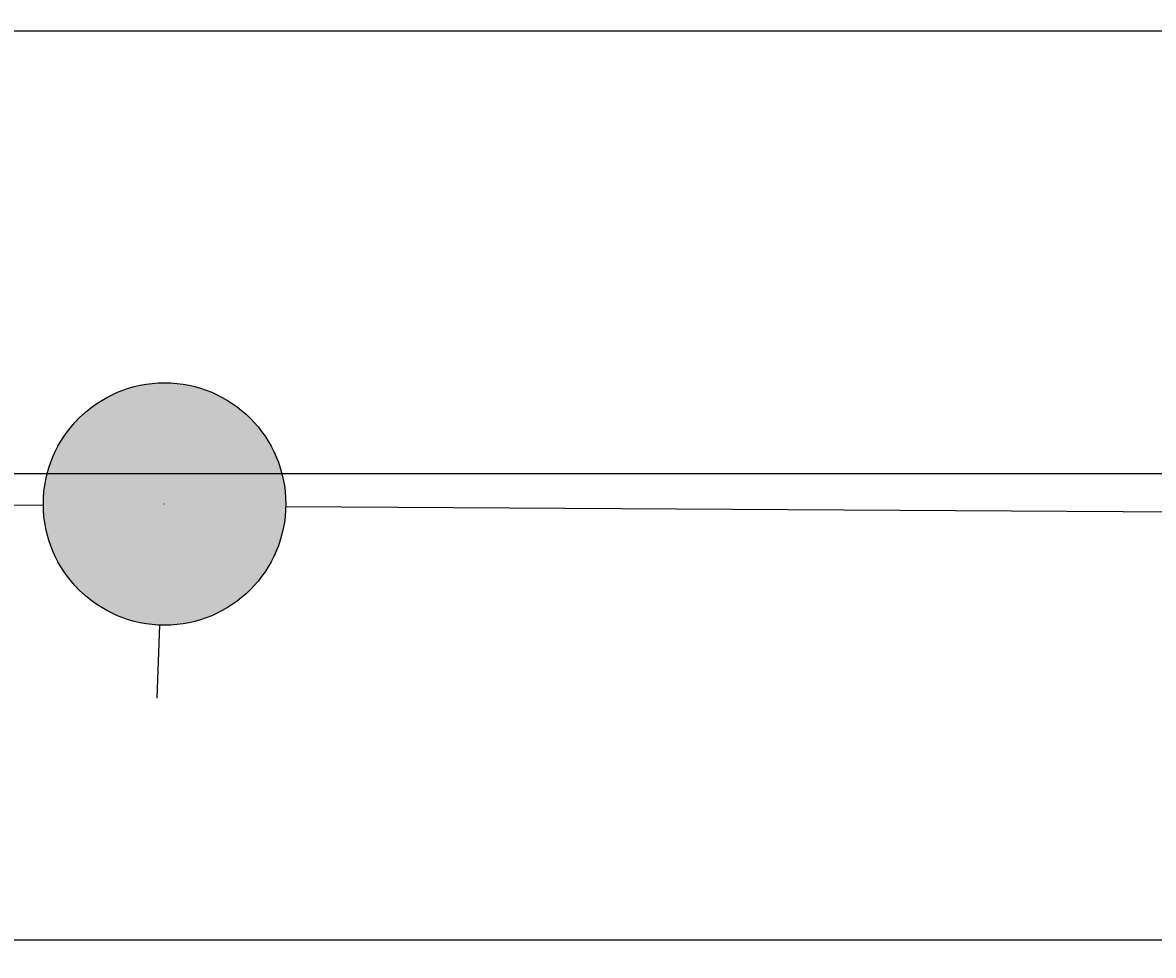
# Model space of a CAD drawing. Units: inches. Extents: x 35362 to 73946, y 43607 to 67532.
# Tile 10 of 134: x 42029 to 43509, y 47688 to 48909. Entities that reach past the tile are written whole.
import ezdxf

# ---------------------------------------------------------------- set-up
doc = ezdxf.new("R2010")
doc.units = ezdxf.units.IN
doc.header["$MEASUREMENT"] = 0
for name, color, linetype, lineweight in [('A-ANNO-DIMS', 2, 'Continuous', 18), ('E-SYMB', 1, 'Continuous', 25), ('E-SYMB-PATT', 1, 'Continuous', 13), ('E-WIRE', 3, 'Continuous', 25)]:
    doc.layers.add(name, color=color, linetype=linetype, lineweight=lineweight)
doc.styles.get("Standard").update_dxf_attribs({"font": 'arial.ttf'})
doc.dimstyles.get("Standard").update_dxf_attribs({"dimtxt": 0.18, "dimasz": 0.18, "dimexe": 0.18, "dimexo": 0.0625, "dimgap": 0.09, "dimtad": 0, "dimtih": 1, "dimtoh": 1, "dimdec": 4, "dimzin": 0, "dimdsep": 46, "dimtxsty": 'Standard', "dimcen": 0.09, "dimadec": 0, "dimazin": 0, "dimtfac": 1, "dimtdec": 4, "dimtofl": 0, "dimtmove": 0, "dimatfit": 3, "dimfxl": 1, "dimtolj": 1, "dimtzin": 0, "dimarcsym": 0})

# ---------------------------------------------------------------- blocks, each defined once
blk = doc.blocks.new('*D21')
at = {"layer": 'A-ANNO-DIMS', "color": 0, "lineweight": -2, "transparency": 16777216}
for p, q in [((42214.5, 48279), (42214.7, 48279)), ((42214.6, 48278.9), (42214.6, 48279.1)), ((42204.8, 48025.4), (42208.5, 48120.3)), ((42204.7, 48025.4), (42204.8, 48025.4))]:
    blk.add_line(p, q, dxfattribs=at)
at = {"layer": 'A-ANNO-DIMS', "color": 0, "transparency": 16777216}
blk.add_solid([(42208.5, 48120.3), (42208.5, 48120.3), (42208.5, 48120.5)], dxfattribs=at)
at = {"layer": 'Defpoints', "color": 0, "transparency": 16777216}
for p in [(42220.8, 48437.5), (42208.5, 48120.5)]:
    blk.add_point(p, dxfattribs=at)
at = {"layer": 'A-ANNO-DIMS', "color": 0, "transparency": 16777216, "insert": (42203.9, 48025.4), "char_height": 0.18, "attachment_point": 5}
blk.add_mtext('\\A1;26X ∅317.2', dxfattribs=at)
blk = doc.blocks.new('*D61')
at = {"layer": 'A-ANNO-DIMS', "color": 0, "lineweight": -2, "transparency": 16777216}
for p, q in [((42214.5, 48279), (42214.7, 48279)), ((42214.6, 48278.9), (42214.6, 48279.1)), ((42204.8, 48025.4), (42208.5, 48120.3)), ((42204.7, 48025.4), (42204.8, 48025.4))]:
    blk.add_line(p, q, dxfattribs=at)
at = {"layer": 'A-ANNO-DIMS', "color": 0, "transparency": 16777216}
blk.add_solid([(42208.5, 48120.3), (42208.5, 48120.3), (42208.5, 48120.5)], dxfattribs=at)
at = {"layer": 'Defpoints', "color": 0, "transparency": 16777216}
for p in [(42220.8, 48437.5), (42208.5, 48120.5)]:
    blk.add_point(p, dxfattribs=at)
at = {"layer": 'A-ANNO-DIMS', "color": 0, "transparency": 16777216, "insert": (42203.9, 48025.4), "char_height": 0.18, "attachment_point": 5}
blk.add_mtext('\\A1;26X ∅317.2', dxfattribs=at)
blk = doc.blocks.new('*D67')
at = {"layer": 'A-ANNO-DIMS', "color": 0, "lineweight": -2, "transparency": 16777216}
for p, q in [((56873.5, 53351.5), (35361.8, 53351.5)), ((35361.9, 53351.3), (35361.9, 49400.9)), ((35361.9, 45450.1), (35361.9, 49400.5)), ((53793.6, 45449.9), (35361.8, 45449.9))]:
    blk.add_line(p, q, dxfattribs=at)
at = {"layer": 'A-ANNO-DIMS', "color": 0, "transparency": 16777216}
for points in [[(35361.9, 53351.3), (35362, 53351.3), (35361.9, 53351.5)], [(35361.9, 45450.1), (35362, 45450.1), (35361.9, 45449.9)]]:
    blk.add_solid(points, dxfattribs=at)
at = {"layer": 'Defpoints', "color": 0, "transparency": 16777216}
for p in [(35361.9, 53351.5), (56873.6, 53351.5), (53793.6, 45449.9)]:
    blk.add_point(p, dxfattribs=at)
at = {"layer": 'A-ANNO-DIMS', "color": 0, "transparency": 16777216, "insert": (35361.9, 49400.7), "char_height": 0.18, "attachment_point": 5}
blk.add_mtext('\\A1;7901.6', dxfattribs=at)
blk = doc.blocks.new('*D87')
at = {"layer": 'A-ANNO-DIMS', "color": 0, "lineweight": -2, "transparency": 16777216}
for p, q in [((52362.5, 48318.3), (35361.8, 48318.3)), ((35361.9, 48318.1), (35361.9, 47931.4)), ((35361.9, 47544.3), (35361.9, 47931)), ((52362.5, 47544.1), (35361.8, 47544.1))]:
    blk.add_line(p, q, dxfattribs=at)
at = {"layer": 'A-ANNO-DIMS', "color": 0, "transparency": 16777216}
for points in [[(35361.9, 48318.1), (35362, 48318.1), (35361.9, 48318.3)], [(35361.9, 47544.3), (35362, 47544.3), (35361.9, 47544.1)]]:
    blk.add_solid(points, dxfattribs=at)
at = {"layer": 'Defpoints', "color": 0, "transparency": 16777216}
for p in [(35361.9, 48318.3), (52362.6, 48318.3), (52362.6, 47544.1)]:
    blk.add_point(p, dxfattribs=at)
at = {"layer": 'A-ANNO-DIMS', "color": 0, "transparency": 16777216, "insert": (35361.9, 47931.2), "char_height": 0.18, "attachment_point": 5}
blk.add_mtext('\\A1;774.1', dxfattribs=at)
blk = doc.blocks.new('*D89')
at = {"layer": 'A-ANNO-DIMS', "color": 0, "lineweight": -2, "transparency": 16777216}
for p, q in [((53707.7, 48897.7), (35361.8, 48897.7)), ((35361.9, 48897.6), (35361.9, 48303.2)), ((35361.9, 47708.4), (35361.9, 48302.8)), ((53707.7, 47708.2), (35361.8, 47708.2))]:
    blk.add_line(p, q, dxfattribs=at)
at = {"layer": 'A-ANNO-DIMS', "color": 0, "transparency": 16777216}
for points in [[(35361.9, 48897.6), (35362, 48897.6), (35361.9, 48897.7)], [(35361.9, 47708.4), (35362, 47708.4), (35361.9, 47708.2)]]:
    blk.add_solid(points, dxfattribs=at)
at = {"layer": 'Defpoints', "color": 0, "transparency": 16777216}
for p in [(53707.8, 48897.7), (35361.9, 47708.2), (53707.8, 47708.2)]:
    blk.add_point(p, dxfattribs=at)
at = {"layer": 'A-ANNO-DIMS', "color": 0, "transparency": 16777216, "insert": (35361.9, 48303), "char_height": 0.18, "attachment_point": 5}
blk.add_mtext('\\A1;1189.5', dxfattribs=at)

msp = doc.modelspace()

# ---------------------------------------------------------------- hatches: boundary and pattern name
at = {"layer": 'E-SYMB-PATT'}
h = msp.add_hatch(color=256, dxfattribs=at)
h.dxf.hatch_style = 1
h.paths.add_polyline_path([(42056.029, 48278.988, 1), (42373.241, 48278.988, 1)])
h = msp.add_hatch(color=256, dxfattribs=at)
h.dxf.hatch_style = 1
h.paths.add_polyline_path([(42373.206, 48275.646), (42056.036, 48277.555, 0.98505792)])

# ---------------------------------------------------------------- linework, layer by layer
at = {"layer": 'E-SYMB'}
msp.add_circle((42214.635, 48278.988), 158.606, dxfattribs=at)
at = {"layer": 'E-WIRE'}
for p, q in [((39894.84, 48290.562), (42056.036, 48277.555)), ((42373.206, 48275.646), (45390.147, 48257.489))]:
    msp.add_line(p, q, dxfattribs=at)

# ---------------------------------------------------------------- dimensions: what is measured, and where the dimension line sits
at = {"layer": 'A-ANNO-DIMS'}
for base, p1, p2, picture, middle in [((35361.949, 53351.529), (53793.638, 45449.894), (56873.602, 53351.529), '*D67', (35361.949, 49400.712)), ((35361.949, 47708.216), (53707.781, 48897.738), (53707.781, 47708.216), '*D89', (35361.949, 48302.977)), ((35361.949, 48318.269), (52362.557, 47544.134), (52362.557, 48318.269), '*D87', (35361.949, 47931.201))]:
    dim = msp.add_linear_dim(base=base, p1=p1, p2=p2, angle=90, dimstyle='Standard', override={"dimdec": 1, "dimlfac": 1, "dimrnd": 0, "dimzin": 0, "dimdsep": 46, "dimlunit": 2}, dxfattribs=at)
    dim.commit()
    dim.dimension.update_dxf_attribs({"geometry": picture, "text_midpoint": middle})
for picture in ['*D21', '*D61']:
    dim = msp.add_diameter_dim_2p(p1=(42220.755, 48437.476), p2=(42208.515, 48120.501), text='26X <>', dimstyle='Standard', override={"dimdec": 1, "dimlfac": 1, "dimrnd": 0, "dimzin": 0, "dimdsep": 46, "dimlunit": 2}, dxfattribs=at)
    dim.commit()
    dim.dimension.update_dxf_attribs({"geometry": picture, "text_midpoint": (42203.912, 48025.408), "dimtype": 163})

doc.saveas('drawing.dxf')
